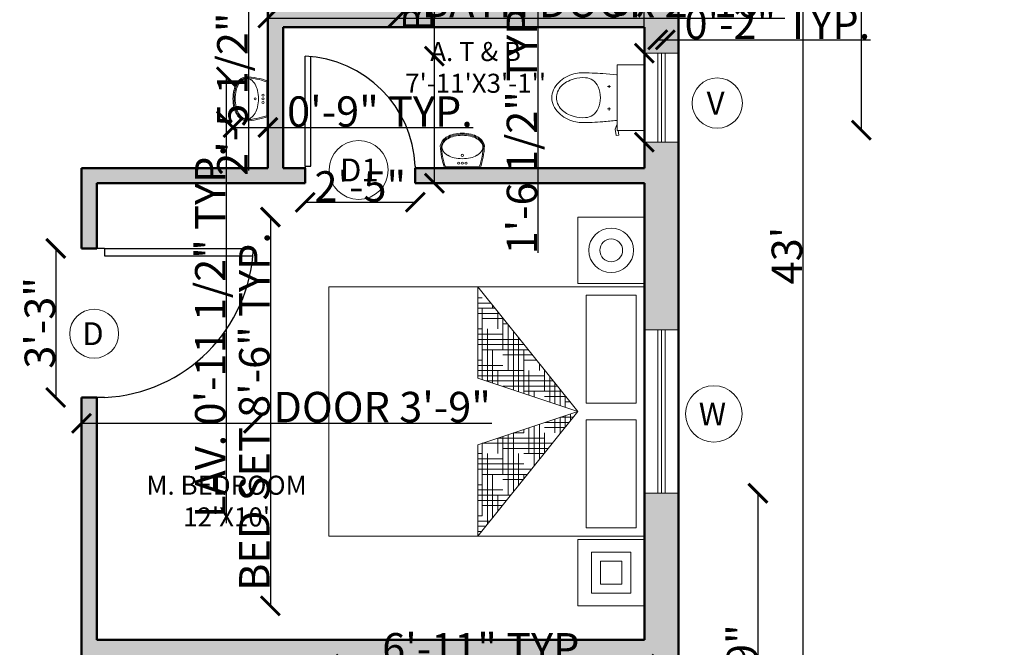
# Model space of a CAD drawing. Units: inches. Extents: x 2169 to 2662, y 1518 to 2151.
# Tile 5 of 6: x 2403 to 2662, y 1751 to 1916. Entities that reach past the tile are written whole.
import ezdxf

# ---------------------------------------------------------------- set-up
doc = ezdxf.new("R2010")
doc.units = ezdxf.units.IN
for name, color, linetype, lineweight in [('A-ANNO-DIMS', 2, 'Continuous', 18), ('A-ANNO-SYMB', 7, 'Continuous', 18), ('A-AREA-IDEN', 7, 'Continuous', 18), ('A-FLOR-FIXT', 9, 'Continuous', 18), ('A-FURN', 8, 'Continuous', 18), ('A-WALL-PATT', 30, 'Continuous', 13), ('Doors', 240, 'Continuous', 30), ('Walls', 7, 'Continuous', 50), ('Windows', 160, 'Continuous', 18)]:
    doc.layers.add(name, color=color, linetype=linetype, lineweight=lineweight)
doc.styles.get("Standard").update_dxf_attribs({"font": 'arial.ttf'})
doc.dimstyles.get("Standard").update_dxf_attribs({"dimtxt": 8, "dimasz": 5, "dimexe": 0.18, "dimexo": 0.0625, "dimgap": 0.09, "dimtad": 1, "dimdec": 1, "dimzin": 0, "dimdsep": 46, "dimlunit": 4, "dimtxsty": 'Standard', "dimblk": 'ARCHTICK', "dimcen": 0.09, "dimse1": 1, "dimse2": 1, "dimadec": 0, "dimazin": 0, "dimtfac": 1, "dimtdec": 1, "dimtofl": 0, "dimtmove": 0, "dimatfit": 3, "dimfxl": 1, "dimtolj": 1, "dimtzin": 0, "dimarcsym": 0})

# ---------------------------------------------------------------- blocks, each defined once
blk = doc.blocks.new('_ArchTick')
at = {"color": 0, "linetype": 'ByBlock', "const_width": 0.15}
blk.add_lwpolyline([(-0.5, -0.5), (0.5, 0.5)], dxfattribs=at)
blk = doc.blocks.new('*D3')
at = {"layer": 'A-ANNO-DIMS', "color": 0, "lineweight": -2, "transparency": 16777216}
blk.add_line((2608.61, 2111.6), (2608.61, 1595.6), dxfattribs=at)
at = {"layer": 'Defpoints', "color": 0, "transparency": 16777216}
for p in [(2575.74, 2111.6), (2575.98, 1595.6), (2608.61, 1595.6)]:
    blk.add_point(p, dxfattribs=at)
at = {"layer": 'A-ANNO-DIMS', "color": 0, "lineweight": -2, "transparency": 16777216, "xscale": 5, "yscale": 5, "zscale": 5}
for p, rotation in [((2608.61, 2111.6), 90), ((2608.61, 1595.6), 270)]:
    blk.add_blockref('_ArchTick', p, dxfattribs=dict(at, rotation=rotation))
at = {"layer": 'A-ANNO-DIMS', "color": 0, "transparency": 16777216, "insert": (2604.43, 1853.6), "char_height": 8, "attachment_point": 5, "rotation": 90}
blk.add_mtext("\\A1;43'", dxfattribs=at)
blk = doc.blocks.new('*X16')
at = {"color": 0}
for p, q in [((20.1875, 14.75), (20.1875, 14.7669)), ((20.199, 14.7812), (20.2772, 14.7812)), ((20.25, 14.8125), (20.2772, 14.8125)), ((20.1487, 14.7188), (20.2772, 14.7188)), ((20.1562, 14.625), (20.1562, 14.7281)), ((20.1739, 14.75), (20.2772, 14.75)), ((20.25, 14.3194), (20.25, 14.75)), ((20.0938, 14.375), (20.0938, 14.6504)), ((20.0984, 14.6562), (20.125, 14.6562)), ((20.1236, 14.6875), (20.25, 14.6875)), ((20.125, 14.5), (20.125, 14.6893)), ((20.0625, 14.2573), (20.0625, 14.6116)), ((20.125, 14.5938), (20.2772, 14.5938)), ((20.2188, 14.3091), (20.2188, 14.625)), ((20.25, 14.625), (20.2772, 14.625)), ((19.9979, 14.5312), (20.2772, 14.5312)), ((20.023, 14.5625), (20.2772, 14.5625)), ((20.0312, 14.2469), (20.0312, 14.5727)), ((19.9476, 14.4688), (20.125, 14.4688)), ((19.9727, 14.5), (20.25, 14.5)), ((20, 14.2366), (20, 14.5)), ((20.1875, 14.2987), (20.1875, 14.5)), ((19.9062, 14.375), (19.9062, 14.4174)), ((19.9225, 14.4375), (20, 14.4375)), ((20.125, 14.4062), (20.2772, 14.4062)), ((20.25, 14.4375), (20.2772, 14.4375)), ((19.875, 14.25), (19.875, 14.3785)), ((19.875, 14.3438), (20.2772, 14.3438)), ((19.9688, 14.2262), (19.9688, 14.375)), ((20, 14.375), (20.2772, 14.375)), ((20.1562, 14.2884), (20.1562, 14.375)), ((19.8125, 14.1744), (19.8125, 14.3008)), ((19.8219, 14.3125), (20.2291, 14.3125)), ((19.8438, 14.1848), (19.8438, 14.3397)), ((19.7716, 14.25), (20, 14.25)), ((19.7812, 14.1641), (19.7812, 14.262)), ((19.7967, 14.2812), (20.125, 14.2812)), ((19.9375, 14.2159), (19.9375, 14.25)), ((19.7213, 14.1875), (19.75, 14.1875)), ((19.7465, 14.2188), (19.875, 14.2188)), ((19.75, 14.1537), (19.75, 14.2231)), ((19.7188, 14.0726), (19.7188, 14.1136)), ((19.7018, 14.0938), (19.7786, 14.0938)), ((19.7269, 14.0625), (19.8728, 14.0625)), ((19.75, 14.0338), (19.75, 14.1032)), ((19.7812, 13.9949), (19.7812, 14.0929)), ((19.8125, 14), (19.8125, 14.0825)), ((19.9062, 13.8396), (19.9062, 14.0514)), ((19.752, 14.0312), (19.875, 14.0312)), ((19.875, 13.8784), (19.875, 14)), ((19.9375, 13.8007), (19.9375, 14.0411)), ((19.9688, 13.875), (19.9688, 14.0307)), ((20, 14), (20, 14.0204)), ((20, 14), (20.0614, 14)), ((20.0625, 13.6454), (20.0625, 13.9996)), ((20.0938, 13.625), (20.0938, 13.9893)), ((19.8275, 13.9375), (20.25, 13.9375)), ((19.875, 13.9688), (20.1557, 13.9688)), ((20.125, 13.75), (20.125, 13.9789)), ((20.1562, 13.875), (20.1562, 13.9686)), ((20.25, 13.5), (20.25, 13.9375)), ((19.8526, 13.9062), (20.125, 13.9062)), ((19.8777, 13.875), (20, 13.875)), ((20.0312, 13.6842), (20.0312, 13.875)), ((20.2188, 13.4511), (20.2188, 13.875)), ((20.25, 13.875), (20.2772, 13.875)), ((20, 13.8125), (20.2772, 13.8125)), ((20.125, 13.8438), (20.2772, 13.8438)), ((19.9532, 13.7812), (20.2772, 13.7812)), ((19.9783, 13.75), (20.25, 13.75)), ((20, 13.723), (20, 13.75)), ((20.0035, 13.7188), (20.125, 13.7188)), ((20.1875, 13.49), (20.1875, 13.75)), ((20.125, 13.6562), (20.2772, 13.6562)), ((20.25, 13.6875), (20.2772, 13.6875)), ((20.0789, 13.625), (20.2772, 13.625)), ((20.104, 13.5938), (20.2772, 13.5938)), ((20.1562, 13.5288), (20.1562, 13.625)), ((20.1292, 13.5625), (20.25, 13.5625)), ((20.2046, 13.4688), (20.2772, 13.4688)), ((20.25, 13.5), (20.2772, 13.5)), ((20.2297, 13.4375), (20.2772, 13.4375)), ((20.2549, 13.4062), (20.2772, 13.4062))]:
    blk.add_line(p, q, dxfattribs=at)
blk = doc.blocks.new('MAT-P13')
for p, q in [((-1.17, 0), (-1.17, -0.4)), ((-1.17, 0), (-0.77, 0)), ((-0.77, 0), (-0.77, -0.4)), ((-0.75, 0), (0.75, 0)), ((-0.75, 0), (-0.75, -1.9)), ((0.75, 0), (0.75, -1.9)), ((0.77, 0), (1.17, 0)), ((0.77, 0), (0.77, -0.4)), ((1.17, 0), (1.17, -0.4)), ((-0.7, -0.05), (-0.7, -0.35)), ((-0.7, -0.05), (-0.05, -0.05)), ((-0.05, -0.35), (-0.05, -0.05)), ((0.05, -0.05), (0.7, -0.05)), ((0.05, -0.35), (0.05, -0.05)), ((0.7, -0.05), (0.7, -0.35)), ((-0.7, -0.35), (-0.05, -0.35)), ((0.05, -0.35), (0.7, -0.35)), ((-1.17, -0.4), (-0.77, -0.4)), ((-0.75, -1.0034), (0, -0.4)), ((0, -0.4), (-0.75, -1.0034)), ((0, -0.4), (-0.2, -1.0034)), ((0, -0.4), (0.2, -1.0034)), ((0, -0.4), (0.75, -1.0034)), ((0.77, -0.4), (1.17, -0.4)), ((-0.75, -1.0034), (-0.2, -1.0034)), ((0.2, -1.0034), (0.75, -1.0034)), ((0.75, -1.9), (-0.75, -1.9))]:
    blk.add_line(p, q)
for points in [[(0.8468, -0.0814), (1.0932, -0.0814), (1.0932, -0.3186), (0.8468, -0.3186)], [(0.9015, -0.1361), (1.0385, -0.1361), (1.0385, -0.2639), (0.9015, -0.2639)]]:
    blk.add_lwpolyline(points, close=True)
for radius in [0.1342, 0.0686]:
    blk.add_circle((-0.97, -0.2), radius)
at = {"xscale": -1, "rotation": 90}
blk.add_blockref('*X16', (14.1285, 19.2738), dxfattribs=at)
blk = doc.blocks.new('toilet-1')
at = {"color": 0, "linetype": 'ByBlock'}
for p, q in [((-0.23, -0.02), (-0.23, -0.2116)), ((0.23, -0.02), (-0.23, -0.02)), ((0.23, -0.02), (0.23, -0.2116)), ((0.2633, -0.1997), (0.23, -0.2044)), ((0.266, -0.2187), (0.2633, -0.1997)), ((-0.23, -0.2116), (0.23, -0.2116)), ((-0.0889, -0.2683), (-0.0697, -0.2683)), ((-0.0793, -0.2587), (-0.0793, -0.2778)), ((0.0889, -0.2683), (0.0698, -0.2683)), ((0.0794, -0.2587), (0.0794, -0.2778)), ((0.1917, -0.2144), (0.2206, -0.225)), ((0.2206, -0.225), (0.266, -0.2187)), ((0, -0.6382), (0, -0.6382))]:
    blk.add_line(p, q, dxfattribs=at)
for centre, radius, start, end in [((3.5272, -0.6239), 3.7093, 173.69251, 175.15926), ((-3.527, -0.624), 3.7093, 4.84131, 6.31706), ((1.7368, -0.4519), 1.9109, 175.76982, 180.37578), ((-0.0312, -0.4465), 0.1114, 113.89968, 145.1485), ((0, -0.5169), 0.1884, 66.09393, 113.90607), ((0.0312, -0.4465), 0.1114, 34.8515, 66.10032), ((-1.7366, -0.4519), 1.9109, 359.62422, 4.23018), ((-0.0408, -0.4398), 0.0996, 145.14967, 175.88096), ((0.0409, -0.4398), 0.0996, 4.11904, 34.85033), ((0.0353, -0.463), 0.2093, 180.37466, 194.33753), ((0.0981, -0.4497), 0.2389, 175.88621, 195.59308), ((-0.098, -0.4497), 0.2389, 344.40692, 4.11379), ((-0.0351, -0.463), 0.2093, 345.6614, 359.62427), ((0.055, -0.458), 0.2297, 194.33532, 209.62204), ((0.0961, -0.4503), 0.2369, 195.59686, 209.37705), ((-0.096, -0.4503), 0.2369, 330.62295, 344.40314), ((-0.0548, -0.458), 0.2297, 330.37879, 345.66551), ((0.0647, -0.4524), 0.2409, 209.62726, 224.54888), ((0.0232, -0.4913), 0.1532, 209.38715, 226.54376), ((0.0178, -0.4986), 0.1751, 224.55199, 245.714), ((0.0152, -0.4997), 0.1416, 226.55015, 246.55272), ((-0.0151, -0.4997), 0.1416, 293.44728, 313.44985), ((-0.0176, -0.4986), 0.1751, 294.28649, 315.4485), ((-0.0231, -0.4913), 0.1532, 313.45624, 330.61285), ((-0.0645, -0.4524), 0.2409, 315.45042, 330.37204), ((0.0004, -0.538), 0.132, 245.58449, 269.87817), ((0, -0.5347), 0.1034, 246.54933, 270.0042), ((0, -0.5347), 0.1034, 269.9958, 293.45067), ((-0.0002, -0.538), 0.132, 270.12162, 294.4153)]:
    blk.add_arc(centre, radius, start, end, dxfattribs=at)
blk = doc.blocks.new('wash-3')
at = {"color": 0, "linetype": 'ByBlock'}
blk.add_line((0.23, -0.015), (-0.23, -0.015), dxfattribs=at)
for centre in [(-0.05, -0.066), (0, -0.066), (0.05, -0.066), (0, -0.172)]:
    blk.add_circle(centre, 0.0148, dxfattribs=at)
for centre, radius, start, end in [((0.69, -0.34), 0.991, 159.941, 177.839), ((0.69, -0.34), 0.976, 160.5399, 177.7326), ((0, -0.61), 0.483, 90, 103.3619), ((0, -0.61), 0.483, 76.6381, 90), ((-0.69, -0.34), 0.976, 2.2674, 19.4601), ((-0.69, -0.34), 0.991, 2.161, 20.059), ((-0.183, -0.286), 0.095, 144.1588, 180), ((-0.096, -0.349), 0.203, 119.8322, 144.1588), ((-0.038, -0.45), 0.319, 103.3619, 119.8322), ((0.038, -0.45), 0.319, 60.1678, 76.6381), ((0.096, -0.349), 0.203, 35.8412, 60.1678), ((0.183, -0.286), 0.095, 0, 35.8412), ((-0.12, -0.265), 0.184, 191.7424, 233.4191), ((-0.12, -0.265), 0.169, 192.3358, 233.361), ((-0.183, -0.286), 0.095, 180, 215.8412), ((-0.096, -0.223), 0.203, 215.8412, 240.1678), ((-0.096, -0.223), 0.217, 234.8176, 240.1678), ((-0.038, -0.122), 0.319, 240.1678, 256.6381), ((0.038, -0.122), 0.319, 283.3619, 299.8322), ((0.096, -0.223), 0.203, 299.8322, 324.1588), ((0.096, -0.223), 0.217, 299.8322, 305.1824), ((0.12, -0.265), 0.169, 306.639, 347.6642), ((0.12, -0.265), 0.184, 306.5809, 348.2576), ((0.183, -0.286), 0.095, 324.1588, 0), ((-0.096, -0.223), 0.232, 234.7719, 240.1678), ((-0.038, -0.122), 0.348, 240.1678, 256.6381), ((-0.038, -0.122), 0.333, 240.1678, 256.6381), ((0, 0.038), 0.513, 256.6381, 270), ((0, 0.038), 0.498, 256.6381, 270), ((0, 0.038), 0.483, 256.6381, 270), ((0, 0.038), 0.483, 270, 283.3619), ((0, 0.038), 0.498, 270, 283.3619), ((0, 0.038), 0.513, 270, 283.3619), ((0.038, -0.122), 0.333, 283.3619, 299.8322), ((0.038, -0.122), 0.348, 283.3619, 299.8322), ((0.096, -0.223), 0.232, 299.8322, 305.2281)]:
    blk.add_arc(centre, radius, start, end, dxfattribs=at)
blk = doc.blocks.new('AP0B05')
for p, q in [((35, 100), (35, 880)), ((75, 100), (75, 878.9)), ((35, 100), (35, -20)), ((815, 100), (815, -20))]:
    blk.add_line(p, q)
blk.add_lwpolyline([(35, 100), (75, 100)])
blk.add_arc((-2.4, 62.6), 818.3, 2.6212, 87.3788)
blk = doc.blocks.new('GLAZING-43IN')
for p, q in [((-21.5, 1), (21.5, 1)), ((-21.5, 0), (21.5, 0)), ((-21.5, -1), (21.5, -1))]:
    blk.add_line(p, q)
blk = doc.blocks.new('GLAZING-SHORT')
for p, q in [((-1, -11.72), (-1, 11.72)), ((0, -11.72), (0, 11.72)), ((1, -11.72), (1, 11.72))]:
    blk.add_line(p, q)
blk = doc.blocks.new('OPENING-TAG-W')
blk.add_circle((0, 0), 7.42)
blk.add_text('W', height=6).set_placement((-3.96, -3))
blk = doc.blocks.new('OPENING-TAG-D')
blk.add_circle((0, 0), 6.43)
blk.add_text('D', height=6).set_placement((-3.13, -3))
blk = doc.blocks.new('OPENING-TAG-V')
blk.add_circle((0, 0), 6.61)
blk.add_text('V', height=6).set_placement((-2.78, -3))
blk = doc.blocks.new('OPENING-TAG-D1')
blk.add_circle((0, 0), 7.74)
blk.add_text('D1', height=6).set_placement((-4.91, -3.01))
blk = doc.blocks.new('*D27')
at = {"layer": 'A-ANNO-DIMS', "color": 0, "lineweight": -2, "transparency": 16777216}
for p, q in [((2566.96, 1906.83), (2566.96, 2079.95)), ((2566.96, 1883.38), (2566.96, 1906.83))]:
    blk.add_line(p, q, dxfattribs=at)
at = {"layer": 'Defpoints', "color": 0, "transparency": 16777216}
for p in [(2566.96, 1906.83), (2570.48, 1906.83), (2570.48, 1883.38)]:
    blk.add_point(p, dxfattribs=at)
at = {"layer": 'A-ANNO-DIMS', "color": 0, "lineweight": -2, "transparency": 16777216, "xscale": 5, "yscale": 5, "zscale": 5}
for p, rotation in [((2566.96, 1906.83), 90), ((2566.96, 1883.38), 270)]:
    blk.add_blockref('_ArchTick', p, dxfattribs=dict(at, rotation=rotation))
at = {"layer": 'A-ANNO-DIMS', "color": 0, "transparency": 16777216, "insert": (2562.73, 1995.89), "char_height": 8, "attachment_point": 5, "rotation": 90}
blk.add_mtext('\\A1;SHORT WINDOW 1\'-11 1/2" TYP.', dxfattribs=at)
blk = doc.blocks.new('*D28')
at = {"layer": 'A-ANNO-DIMS', "color": 0, "lineweight": -2, "transparency": 16777216}
for p, q in [((2570.48, 1910.34), (2572.48, 1910.34)), ((2572.48, 1910.34), (2626.42, 1910.34))]:
    blk.add_line(p, q, dxfattribs=at)
at = {"layer": 'Defpoints', "color": 0, "transparency": 16777216}
for p in [(2572.48, 1910.34), (2570.48, 1906.83), (2572.48, 1906.83)]:
    blk.add_point(p, dxfattribs=at)
at = {"layer": 'A-ANNO-DIMS', "color": 0, "lineweight": -2, "transparency": 16777216, "xscale": 5, "yscale": 5, "zscale": 5, "rotation": 180}
blk.add_blockref('_ArchTick', (2570.48, 1910.34), dxfattribs=at)
at = {"layer": 'A-ANNO-DIMS', "color": 0, "lineweight": -2, "transparency": 16777216, "xscale": 5, "yscale": 5, "zscale": 5}
blk.add_blockref('_ArchTick', (2572.48, 1910.34), dxfattribs=at)
at = {"layer": 'A-ANNO-DIMS', "color": 0, "transparency": 16777216, "insert": (2601.95, 1914.52), "char_height": 8, "attachment_point": 5}
blk.add_mtext('\\A1;0\'-2" TYP.', dxfattribs=at)
blk = doc.blocks.new('*D33')
at = {"layer": 'A-ANNO-DIMS', "color": 0, "lineweight": -2, "transparency": 16777216}
for p, q in [((2467.98, 1916.03), (2502.05, 1916.03)), ((2502.05, 1916.03), (2603.9, 1916.03))]:
    blk.add_line(p, q, dxfattribs=at)
at = {"layer": 'Defpoints', "color": 0, "transparency": 16777216}
for p in [(2467.98, 1921.14), (2502.05, 1921.14), (2502.05, 1916.03)]:
    blk.add_point(p, dxfattribs=at)
at = {"layer": 'A-ANNO-DIMS', "color": 0, "lineweight": -2, "transparency": 16777216, "xscale": 5, "yscale": 5, "zscale": 5, "rotation": 180}
blk.add_blockref('_ArchTick', (2467.98, 1916.03), dxfattribs=at)
at = {"layer": 'A-ANNO-DIMS', "color": 0, "lineweight": -2, "transparency": 16777216, "xscale": 5, "yscale": 5, "zscale": 5}
blk.add_blockref('_ArchTick', (2502.05, 1916.03), dxfattribs=at)
at = {"layer": 'A-ANNO-DIMS', "color": 0, "transparency": 16777216, "insert": (2555.47, 1920.26), "char_height": 8, "attachment_point": 5}
blk.add_mtext('\\A1;BATH DOOR 2\'-10"', dxfattribs=at)
blk = doc.blocks.new('*D34')
at = {"layer": 'A-ANNO-DIMS', "color": 0, "lineweight": -2, "transparency": 16777216}
for p, q in [((2462.86, 1950.67), (2462.86, 1921.14)), ((2462.86, 1921.14), (2462.86, 1875.92))]:
    blk.add_line(p, q, dxfattribs=at)
at = {"layer": 'Defpoints', "color": 0, "transparency": 16777216}
for p in [(2467.98, 1950.67), (2462.86, 1921.14), (2467.98, 1921.14)]:
    blk.add_point(p, dxfattribs=at)
at = {"layer": 'A-ANNO-DIMS', "color": 0, "lineweight": -2, "transparency": 16777216, "xscale": 5, "yscale": 5, "zscale": 5}
for p, rotation in [((2462.86, 1950.67), 90), ((2462.86, 1921.14), 270)]:
    blk.add_blockref('_ArchTick', p, dxfattribs=dict(at, rotation=rotation))
at = {"layer": 'A-ANNO-DIMS', "color": 0, "transparency": 16777216, "insert": (2458.64, 1896.03), "char_height": 8, "attachment_point": 5, "rotation": 90}
blk.add_mtext('\\A1;2\'-5 1/2"', dxfattribs=at)
blk = doc.blocks.new('*D35')
at = {"layer": 'A-ANNO-DIMS', "color": 0, "lineweight": -2, "transparency": 16777216}
for p, q in [((2418.98, 1809.52), (2464.19, 1809.52)), ((2464.19, 1809.52), (2526.87, 1809.52))]:
    blk.add_line(p, q, dxfattribs=at)
at = {"layer": 'Defpoints', "color": 0, "transparency": 16777216}
for p in [(2418.98, 1816.31), (2464.19, 1816.31), (2464.19, 1809.52)]:
    blk.add_point(p, dxfattribs=at)
at = {"layer": 'A-ANNO-DIMS', "color": 0, "lineweight": -2, "transparency": 16777216, "xscale": 5, "yscale": 5, "zscale": 5, "rotation": 180}
blk.add_blockref('_ArchTick', (2418.98, 1809.52), dxfattribs=at)
at = {"layer": 'A-ANNO-DIMS', "color": 0, "lineweight": -2, "transparency": 16777216, "xscale": 5, "yscale": 5, "zscale": 5}
blk.add_blockref('_ArchTick', (2464.19, 1809.52), dxfattribs=at)
at = {"layer": 'A-ANNO-DIMS', "color": 0, "transparency": 16777216, "insert": (2498.03, 1813.76), "char_height": 8, "attachment_point": 5}
blk.add_mtext('\\A1;DOOR 3\'-9"', dxfattribs=at)
blk = doc.blocks.new('*D36')
at = {"layer": 'A-ANNO-DIMS', "color": 0, "lineweight": -2, "transparency": 16777216}
blk.add_line((2412.19, 1855.49), (2412.19, 1816.31), dxfattribs=at)
at = {"layer": 'Defpoints', "color": 0, "transparency": 16777216}
for p in [(2418.98, 1855.49), (2412.19, 1816.31), (2418.98, 1816.31)]:
    blk.add_point(p, dxfattribs=at)
at = {"layer": 'A-ANNO-DIMS', "color": 0, "lineweight": -2, "transparency": 16777216, "xscale": 5, "yscale": 5, "zscale": 5}
for p, rotation in [((2412.19, 1855.49), 90), ((2412.19, 1816.31), 270)]:
    blk.add_blockref('_ArchTick', p, dxfattribs=dict(at, rotation=rotation))
at = {"layer": 'A-ANNO-DIMS', "color": 0, "transparency": 16777216, "insert": (2408.02, 1835.9), "char_height": 8, "attachment_point": 5, "rotation": 90}
blk.add_mtext('\\A1;3\'-3"', dxfattribs=at)
blk = doc.blocks.new('*D39')
at = {"layer": 'A-ANNO-DIMS', "color": 0, "lineweight": -2, "transparency": 16777216}
for p, q in [((2511.76, 1906), (2511.76, 2020.27)), ((2511.76, 1872.6), (2511.76, 1906))]:
    blk.add_line(p, q, dxfattribs=at)
at = {"layer": 'Defpoints', "color": 0, "transparency": 16777216}
for p in [(2506.75, 1906), (2511.76, 1906), (2506.75, 1872.6)]:
    blk.add_point(p, dxfattribs=at)
at = {"layer": 'A-ANNO-DIMS', "color": 0, "lineweight": -2, "transparency": 16777216, "xscale": 5, "yscale": 5, "zscale": 5}
for p, rotation in [((2511.76, 1906), 90), ((2511.76, 1872.6), 270)]:
    blk.add_blockref('_ArchTick', p, dxfattribs=dict(at, rotation=rotation))
at = {"layer": 'A-ANNO-DIMS', "color": 0, "transparency": 16777216, "insert": (2507.53, 1965.63), "char_height": 8, "attachment_point": 5, "rotation": 90}
blk.add_mtext('\\A1;BATH DOOR 2\'-9 1/2"', dxfattribs=at)
blk = doc.blocks.new('*D40')
at = {"layer": 'A-ANNO-DIMS', "color": 0, "lineweight": -2, "transparency": 16777216}
blk.add_line((2477.81, 1867.6), (2506.75, 1867.6), dxfattribs=at)
at = {"layer": 'Defpoints', "color": 0, "transparency": 16777216}
for p in [(2477.81, 1872.6), (2506.75, 1872.6), (2506.75, 1867.6)]:
    blk.add_point(p, dxfattribs=at)
at = {"layer": 'A-ANNO-DIMS', "color": 0, "lineweight": -2, "transparency": 16777216, "xscale": 5, "yscale": 5, "zscale": 5, "rotation": 180}
blk.add_blockref('_ArchTick', (2477.81, 1867.6), dxfattribs=at)
at = {"layer": 'A-ANNO-DIMS', "color": 0, "lineweight": -2, "transparency": 16777216, "xscale": 5, "yscale": 5, "zscale": 5}
blk.add_blockref('_ArchTick', (2506.75, 1867.6), dxfattribs=at)
at = {"layer": 'A-ANNO-DIMS', "color": 0, "transparency": 16777216, "insert": (2492.28, 1871.77), "char_height": 8, "attachment_point": 5}
blk.add_mtext('\\A1;2\'-5"', dxfattribs=at)
blk = doc.blocks.new('*D43')
at = {"layer": 'A-ANNO-DIMS', "color": 0, "lineweight": -2, "transparency": 16777216}
blk.add_line((2468.65, 1863.71), (2468.65, 1761.5), dxfattribs=at)
at = {"layer": 'Defpoints', "color": 0, "transparency": 16777216}
for p in [(2483.98, 1863.71), (2468.65, 1761.5), (2483.98, 1761.5)]:
    blk.add_point(p, dxfattribs=at)
at = {"layer": 'A-ANNO-DIMS', "color": 0, "lineweight": -2, "transparency": 16777216, "xscale": 5, "yscale": 5, "zscale": 5}
for p, rotation in [((2468.65, 1863.71), 90), ((2468.65, 1761.5), 270)]:
    blk.add_blockref('_ArchTick', p, dxfattribs=dict(at, rotation=rotation))
at = {"layer": 'A-ANNO-DIMS', "color": 0, "transparency": 16777216, "insert": (2464.42, 1812.6), "char_height": 8, "attachment_point": 5, "rotation": 90}
blk.add_mtext('\\A1;BED SET 8\'-6" TYP.', dxfattribs=at)
blk = doc.blocks.new('*D44')
at = {"layer": 'A-ANNO-DIMS', "color": 0, "lineweight": -2, "transparency": 16777216}
blk.add_line((2483.98, 1746.17), (2566.98, 1746.17), dxfattribs=at)
at = {"layer": 'Defpoints', "color": 0, "transparency": 16777216}
for p in [(2483.98, 1761.5), (2566.98, 1761.5), (2566.98, 1746.17)]:
    blk.add_point(p, dxfattribs=at)
at = {"layer": 'A-ANNO-DIMS', "color": 0, "lineweight": -2, "transparency": 16777216, "xscale": 5, "yscale": 5, "zscale": 5, "rotation": 180}
blk.add_blockref('_ArchTick', (2483.98, 1746.17), dxfattribs=at)
at = {"layer": 'A-ANNO-DIMS', "color": 0, "lineweight": -2, "transparency": 16777216, "xscale": 5, "yscale": 5, "zscale": 5}
blk.add_blockref('_ArchTick', (2566.98, 1746.17), dxfattribs=at)
at = {"layer": 'A-ANNO-DIMS', "color": 0, "transparency": 16777216, "insert": (2525.48, 1750.34), "char_height": 8, "attachment_point": 5}
blk.add_mtext('\\A1;6\'-11" TYP.', dxfattribs=at)
blk = doc.blocks.new('*D49')
at = {"layer": 'A-ANNO-DIMS', "color": 0, "lineweight": -2, "transparency": 16777216}
for p, q in [((2542.64, 1922.5), (2566.98, 1922.5)), ((2566.98, 1922.5), (2661.61, 1922.5))]:
    blk.add_line(p, q, dxfattribs=at)
at = {"layer": 'Defpoints', "color": 0, "transparency": 16777216}
for p in [(2542.64, 1926.15), (2566.98, 1926.15), (2566.98, 1922.5)]:
    blk.add_point(p, dxfattribs=at)
at = {"layer": 'A-ANNO-DIMS', "color": 0, "lineweight": -2, "transparency": 16777216, "xscale": 5, "yscale": 5, "zscale": 5, "rotation": 180}
blk.add_blockref('_ArchTick', (2542.64, 1922.5), dxfattribs=at)
at = {"layer": 'A-ANNO-DIMS', "color": 0, "lineweight": -2, "transparency": 16777216, "xscale": 5, "yscale": 5, "zscale": 5}
blk.add_blockref('_ArchTick', (2566.98, 1922.5), dxfattribs=at)
at = {"layer": 'A-ANNO-DIMS', "color": 0, "transparency": 16777216, "insert": (2616.79, 1926.72), "char_height": 8, "attachment_point": 5}
blk.add_mtext('\\A1;WC 2\'-0 1/2" TYP.', dxfattribs=at)
blk = doc.blocks.new('*D50')
at = {"layer": 'A-ANNO-DIMS', "color": 0, "lineweight": -2, "transparency": 16777216}
for p, q in [((2538.99, 1944.71), (2538.99, 1926.15)), ((2538.99, 1926.15), (2538.99, 1854.31))]:
    blk.add_line(p, q, dxfattribs=at)
at = {"layer": 'Defpoints', "color": 0, "transparency": 16777216}
for p in [(2542.64, 1944.71), (2538.99, 1926.15), (2542.64, 1926.15)]:
    blk.add_point(p, dxfattribs=at)
at = {"layer": 'A-ANNO-DIMS', "color": 0, "lineweight": -2, "transparency": 16777216, "xscale": 5, "yscale": 5, "zscale": 5}
for p, rotation in [((2538.99, 1944.71), 90), ((2538.99, 1926.15), 270)]:
    blk.add_blockref('_ArchTick', p, dxfattribs=dict(at, rotation=rotation))
at = {"layer": 'A-ANNO-DIMS', "color": 0, "transparency": 16777216, "insert": (2534.77, 1887.73), "char_height": 8, "attachment_point": 5, "rotation": 90}
blk.add_mtext('\\A1;1\'-6 1/2" TYP.', dxfattribs=at)
blk = doc.blocks.new('*D51')
at = {"layer": 'A-ANNO-DIMS', "color": 0, "lineweight": -2, "transparency": 16777216}
for p, q in [((2457.05, 1900.61), (2457.05, 1889.01)), ((2457.05, 1889.01), (2457.05, 1783.23))]:
    blk.add_line(p, q, dxfattribs=at)
at = {"layer": 'Defpoints', "color": 0, "transparency": 16777216}
for p in [(2458.79, 1900.61), (2457.05, 1889.01), (2458.79, 1889.01)]:
    blk.add_point(p, dxfattribs=at)
at = {"layer": 'A-ANNO-DIMS', "color": 0, "lineweight": -2, "transparency": 16777216, "xscale": 5, "yscale": 5, "zscale": 5}
for p, rotation in [((2457.05, 1900.61), 90), ((2457.05, 1889.01), 270)]:
    blk.add_blockref('_ArchTick', p, dxfattribs=dict(at, rotation=rotation))
at = {"layer": 'A-ANNO-DIMS', "color": 0, "transparency": 16777216, "insert": (2452.83, 1833.62), "char_height": 8, "attachment_point": 5, "rotation": 90}
blk.add_mtext('\\A1;LAV. 0\'-11 1/2" TYP.', dxfattribs=at)
blk = doc.blocks.new('*D52')
at = {"layer": 'A-ANNO-DIMS', "color": 0, "lineweight": -2, "transparency": 16777216}
for p, q in [((2458.79, 1887.27), (2467.98, 1887.27)), ((2467.98, 1887.27), (2521.92, 1887.27))]:
    blk.add_line(p, q, dxfattribs=at)
at = {"layer": 'Defpoints', "color": 0, "transparency": 16777216}
for p in [(2458.79, 1889.01), (2467.98, 1889.01), (2467.98, 1887.27)]:
    blk.add_point(p, dxfattribs=at)
at = {"layer": 'A-ANNO-DIMS', "color": 0, "lineweight": -2, "transparency": 16777216, "xscale": 5, "yscale": 5, "zscale": 5, "rotation": 180}
blk.add_blockref('_ArchTick', (2458.79, 1887.27), dxfattribs=at)
at = {"layer": 'A-ANNO-DIMS', "color": 0, "lineweight": -2, "transparency": 16777216, "xscale": 5, "yscale": 5, "zscale": 5}
blk.add_blockref('_ArchTick', (2467.98, 1887.27), dxfattribs=at)
at = {"layer": 'A-ANNO-DIMS', "color": 0, "transparency": 16777216, "insert": (2497.45, 1891.45), "char_height": 8, "attachment_point": 5}
blk.add_mtext('\\A1;0\'-9" TYP.', dxfattribs=at)
blk = doc.blocks.new('*D55')
at = {"layer": 'A-ANNO-DIMS', "color": 0, "lineweight": -2, "transparency": 16777216}
blk.add_line((2462.45, 2141.45), (2522.45, 2141.45), dxfattribs=at)
at = {"layer": 'Defpoints', "color": 0, "transparency": 16777216}
for p in [(2522.45, 2141.45), (2462.45, 1604.6), (2522.45, 1604.6)]:
    blk.add_point(p, dxfattribs=at)
at = {"layer": 'A-ANNO-DIMS', "color": 0, "lineweight": -2, "transparency": 16777216, "xscale": 5, "yscale": 5, "zscale": 5, "rotation": 180}
blk.add_blockref('_ArchTick', (2462.45, 2141.45), dxfattribs=at)
at = {"layer": 'A-ANNO-DIMS', "color": 0, "lineweight": -2, "transparency": 16777216, "xscale": 5, "yscale": 5, "zscale": 5}
blk.add_blockref('_ArchTick', (2522.45, 2141.45), dxfattribs=at)
at = {"layer": 'A-ANNO-DIMS', "color": 0, "transparency": 16777216, "insert": (2492.45, 2145.63), "char_height": 8, "attachment_point": 5}
blk.add_mtext('\\A1;5\'-0"', dxfattribs=at)
blk = doc.blocks.new('*D62')
at = {"layer": 'A-ANNO-DIMS', "color": 0, "lineweight": -2, "transparency": 16777216}
blk.add_line((2596.83, 1791.1), (2596.83, 1698.1), dxfattribs=at)
at = {"layer": 'Defpoints', "color": 0, "transparency": 16777216}
for p in [(2566.98, 1791.1), (2566.98, 1698.1), (2596.83, 1698.1)]:
    blk.add_point(p, dxfattribs=at)
at = {"layer": 'A-ANNO-DIMS', "color": 0, "lineweight": -2, "transparency": 16777216, "xscale": 5, "yscale": 5, "zscale": 5}
for p, rotation in [((2596.83, 1791.1), 90), ((2596.83, 1698.1), 270)]:
    blk.add_blockref('_ArchTick', p, dxfattribs=dict(at, rotation=rotation))
at = {"layer": 'A-ANNO-DIMS', "color": 0, "transparency": 16777216, "insert": (2592.65, 1744.6), "char_height": 8, "attachment_point": 5, "rotation": 90}
blk.add_mtext('\\A1;7\'-9"', dxfattribs=at)
blk = doc.blocks.new('*D73')
at = {"layer": 'A-ANNO-DIMS', "color": 0, "lineweight": -2, "transparency": 16777216}
blk.add_line((2624.02, 1886.6), (2624.02, 1978.6), dxfattribs=at)
at = {"layer": 'Defpoints', "color": 0, "transparency": 16777216}
for p in [(2369.77, 1978.6), (2624.02, 1978.6), (2370.48, 1886.6)]:
    blk.add_point(p, dxfattribs=at)
at = {"layer": 'A-ANNO-DIMS', "color": 0, "lineweight": -2, "transparency": 16777216, "xscale": 5, "yscale": 5, "zscale": 5}
for p, rotation in [((2624.02, 1978.6), 90), ((2624.02, 1886.6), 270)]:
    blk.add_blockref('_ArchTick', p, dxfattribs=dict(at, rotation=rotation))
at = {"layer": 'A-ANNO-DIMS', "color": 0, "transparency": 16777216, "insert": (2619.84, 1932.6), "char_height": 8, "attachment_point": 5, "rotation": 90}
blk.add_mtext('\\A1;7\'-8"', dxfattribs=at)
blk = doc.blocks.new('*D77')
at = {"layer": 'A-ANNO-DIMS', "color": 0, "lineweight": -2, "transparency": 16777216}
blk.add_line((2566.98, 1525.75), (2523.78, 1525.75), dxfattribs=at)
at = {"layer": 'Defpoints', "color": 0, "transparency": 16777216}
for p in [(2523.78, 1876.6), (2566.98, 1876.6), (2523.78, 1525.75)]:
    blk.add_point(p, dxfattribs=at)
at = {"layer": 'A-ANNO-DIMS', "color": 0, "lineweight": -2, "transparency": 16777216, "xscale": 5, "yscale": 5, "zscale": 5, "rotation": 180}
blk.add_blockref('_ArchTick', (2523.78, 1525.75), dxfattribs=at)
at = {"layer": 'A-ANNO-DIMS', "color": 0, "lineweight": -2, "transparency": 16777216, "xscale": 5, "yscale": 5, "zscale": 5}
blk.add_blockref('_ArchTick', (2566.98, 1525.75), dxfattribs=at)
at = {"layer": 'A-ANNO-DIMS', "color": 0, "transparency": 16777216, "insert": (2545.38, 1529.93), "char_height": 8, "attachment_point": 5}
blk.add_mtext('\\A1;3\'-7"', dxfattribs=at)
blk = doc.blocks.new('*D78')
at = {"layer": 'A-ANNO-DIMS', "color": 0, "lineweight": -2, "transparency": 16777216}
for p, q in [((2393.13, 1748.6), (2393.13, 1792.94)), ((2393.13, 1729.93), (2393.13, 1748.6))]:
    blk.add_line(p, q, dxfattribs=at)
at = {"layer": 'Defpoints', "color": 0, "transparency": 16777216}
for p in [(2393.13, 1748.6), (2422.98, 1748.6), (2422.98, 1729.93)]:
    blk.add_point(p, dxfattribs=at)
at = {"layer": 'A-ANNO-DIMS', "color": 0, "lineweight": -2, "transparency": 16777216, "xscale": 5, "yscale": 5, "zscale": 5}
for p, rotation in [((2393.13, 1748.6), 90), ((2393.13, 1729.93), 270)]:
    blk.add_blockref('_ArchTick', p, dxfattribs=dict(at, rotation=rotation))
at = {"layer": 'A-ANNO-DIMS', "color": 0, "transparency": 16777216, "insert": (2388.9, 1773.27), "char_height": 8, "attachment_point": 5, "rotation": 90}
blk.add_mtext('\\A1;1\'-6 1/2"', dxfattribs=at)
blk = doc.blocks.new('*D79')
at = {"layer": 'A-ANNO-DIMS', "color": 0, "lineweight": -2, "transparency": 16777216}
for p, q in [((2393.13, 1872.6), (2393.13, 1898.3)), ((2393.13, 1855.49), (2393.13, 1872.6))]:
    blk.add_line(p, q, dxfattribs=at)
at = {"layer": 'Defpoints', "color": 0, "transparency": 16777216}
for p in [(2393.13, 1872.6), (2422.98, 1872.6), (2422.98, 1855.49)]:
    blk.add_point(p, dxfattribs=at)
at = {"layer": 'A-ANNO-DIMS', "color": 0, "lineweight": -2, "transparency": 16777216, "xscale": 5, "yscale": 5, "zscale": 5}
for p, rotation in [((2393.13, 1872.6), 90), ((2393.13, 1855.49), 270)]:
    blk.add_blockref('_ArchTick', p, dxfattribs=dict(at, rotation=rotation))
at = {"layer": 'A-ANNO-DIMS', "color": 0, "transparency": 16777216, "insert": (2388.95, 1887.95), "char_height": 8, "attachment_point": 5, "rotation": 90}
blk.add_mtext('\\A1;1\'-5"', dxfattribs=at)
blk = doc.blocks.new('*D86')
at = {"layer": 'A-ANNO-DIMS', "color": 0, "lineweight": -2, "transparency": 16777216}
for p, q in [((2471.98, 1525.75), (2477.81, 1525.75)), ((2477.81, 1525.75), (2504.25, 1525.75))]:
    blk.add_line(p, q, dxfattribs=at)
at = {"layer": 'Defpoints', "color": 0, "transparency": 16777216}
for p in [(2471.98, 1876.6), (2477.81, 1876.6), (2477.81, 1525.75)]:
    blk.add_point(p, dxfattribs=at)
at = {"layer": 'A-ANNO-DIMS', "color": 0, "lineweight": -2, "transparency": 16777216, "xscale": 5, "yscale": 5, "zscale": 5, "rotation": 180}
blk.add_blockref('_ArchTick', (2471.98, 1525.75), dxfattribs=at)
at = {"layer": 'A-ANNO-DIMS', "color": 0, "lineweight": -2, "transparency": 16777216, "xscale": 5, "yscale": 5, "zscale": 5}
blk.add_blockref('_ArchTick', (2477.81, 1525.75), dxfattribs=at)
at = {"layer": 'A-ANNO-DIMS', "color": 0, "transparency": 16777216, "insert": (2493.53, 1529.93), "char_height": 8, "attachment_point": 5}
blk.add_mtext('\\A1;0\'-6"', dxfattribs=at)

msp = doc.modelspace()

# ---------------------------------------------------------------- hatches: boundary and pattern name
at = {"layer": 'A-WALL-PATT', "transparency": 33554585}
h = msp.add_hatch(color=256, dxfattribs=at)
h.dxf.hatch_style = 1
h.paths.add_polyline_path([(2575.98, 2111.6), (2263.98, 2111.6), (2263.98, 2066.68), (2272.98, 2066.68), (2272.98, 2102.6), (2418.98, 2102.6), (2418.98, 1982.6), (2413.75, 1982.6), (2413.75, 1978.6), (2418.98, 1978.6), (2418.98, 1954.6), (2429.26, 1954.6), (2429.26, 1958.6), (2422.98, 1958.6), (2422.98, 2102.6), (2566.98, 2102.6), (2566.98, 2052.1), (2575.98, 2052.1)])
h.paths.add_polyline_path([(2575.98, 2009.1), (2566.98, 2009.1), (2566.98, 1997.84), (2566.98, 1958.6), (2467.98, 1958.6), (2467.98, 1950.67), (2471.98, 1950.67), (2471.98, 1954.6), (2566.98, 1954.6), (2566.98, 1947.83), (2575.98, 1947.83)])
h.paths.add_polyline_path([(2272.98, 2023.68), (2263.98, 2023.68), (2263.98, 1944.7), (2272.98, 1944.7), (2272.98, 1978.6), (2369.77, 1978.6), (2369.77, 1982.6), (2272.98, 1982.6)])
h.paths.add_polyline_path([(2272.98, 1882.6), (2370.48, 1882.6), (2370.48, 1886.6), (2272.98, 1886.6), (2272.98, 1921.26), (2263.98, 1921.26), (2263.98, 1841.55), (2272.98, 1841.55)])
h.paths.add_polyline_path([(2272.98, 1798.55), (2263.98, 1798.55), (2263.98, 1689.49), (2272.98, 1689.49)])
h.paths.add_polyline_path([(2272.98, 1646.49), (2263.98, 1646.49), (2263.98, 1595.6), (2281.85, 1595.6), (2281.85, 1604.6), (2272.98, 1604.6)])
h.paths.add_polyline_path([(2342.72, 1600.02), (2342.72, 1604.6), (2324.85, 1604.6), (2324.85, 1595.6), (2342.72, 1595.6)])
h.paths.add_polyline_path([(2462.45, 1604.6), (2408.92, 1604.6), (2408.92, 1595.6), (2462.45, 1595.6)])
h.paths.add_polyline_path([(2422.98, 1689.75), (2418.98, 1689.75), (2418.98, 1604.6), (2422.98, 1604.6)])
h.paths.add_polyline_path([(2575.98, 1655.1), (2566.98, 1655.1), (2566.98, 1643.84), (2566.98, 1604.6), (2522.45, 1604.6), (2522.45, 1595.6), (2575.98, 1595.6)])
h.paths.add_polyline_path([(2575.98, 1791.1), (2566.98, 1791.1), (2566.98, 1752.6), (2422.98, 1752.6), (2422.98, 1816.31), (2418.98, 1816.31), (2418.98, 1729.93), (2422.98, 1729.93), (2422.98, 1748.6), (2566.98, 1748.6), (2566.98, 1698.1), (2575.98, 1698.1)])
h.paths.add_polyline_path([(2575.98, 1883.38), (2566.98, 1883.38), (2566.98, 1876.6), (2506.75, 1876.6), (2506.75, 1872.6), (2566.98, 1872.6), (2566.98, 1834.1), (2575.98, 1834.1)])
h.paths.add_polyline_path([(2477.81, 1876.6), (2471.98, 1876.6), (2471.98, 1913.6), (2566.98, 1913.6), (2566.98, 1906.83), (2575.98, 1906.83), (2575.98, 1924.38), (2566.98, 1924.38), (2566.98, 1917.6), (2471.98, 1917.6), (2471.98, 1921.14), (2467.98, 1921.14), (2467.98, 1876.6), (2418.98, 1876.6), (2418.98, 1855.49), (2422.98, 1855.49), (2422.98, 1872.6), (2477.81, 1872.6)])

# ---------------------------------------------------------------- linework, layer by layer
at = {"layer": 'Walls'}
for p, q in [((2575.98, 2111.6), (2575.98, 1595.6)), ((2467.98, 1921.14), (2467.98, 1876.6)), ((2471.98, 1913.6), (2566.98, 1913.6)), ((2471.98, 1913.6), (2471.98, 1876.6)), ((2566.98, 1913.6), (2566.98, 1876.6)), ((2418.98, 1876.6), (2467.98, 1876.6)), ((2418.98, 1876.6), (2418.98, 1855.49)), ((2471.98, 1876.6), (2477.81, 1876.6)), ((2477.81, 1872.6), (2477.81, 1876.6)), ((2506.75, 1872.6), (2506.75, 1876.6)), ((2506.75, 1876.6), (2566.98, 1876.6)), ((2422.98, 1872.6), (2477.81, 1872.6)), ((2422.98, 1872.6), (2422.98, 1855.49)), ((2506.75, 1872.6), (2566.98, 1872.6)), ((2566.98, 1872.6), (2566.98, 1752.6)), ((2418.98, 1855.49), (2422.98, 1855.49)), ((2418.98, 1816.31), (2422.98, 1816.31)), ((2418.98, 1816.31), (2418.98, 1729.93)), ((2422.98, 1816.31), (2422.98, 1752.6)), ((2422.98, 1752.6), (2566.98, 1752.6))]:
    msp.add_line(p, q, dxfattribs=at)
at = {"layer": 'Windows'}
for points in [[(2566.98, 1883.38), (2566.98, 1906.83), (2575.98, 1906.83), (2575.98, 1883.38)], [(2566.98, 1791.1), (2566.98, 1834.1), (2575.98, 1834.1), (2575.98, 1791.1)]]:
    msp.add_lwpolyline(points, close=True, dxfattribs=at)

# ---------------------------------------------------------------- block references
at = {"layer": 'A-ANNO-SYMB'}
for name, p in [('OPENING-TAG-V', (2586.13, 1893.67)), ('OPENING-TAG-D1', (2491.85, 1876.11)), ('OPENING-TAG-D', (2422.3, 1833.05)), ('OPENING-TAG-W', (2585.24, 1811.95))]:
    msp.add_blockref(name, p, dxfattribs=at)
at = {"layer": 'A-FLOR-FIXT'}
for name, p, xscale, yscale, zscale, rotation in [('toilet-1', (2567.72, 1895.1), 37.43636210933806, 37.43636210933806, 37.43636210933806, 270), ('wash-3', (2467.98, 1894.81), 19.33450794020463, 19.33450794020463, 19.33450794020463, 270), ('wash-3', (2519.12, 1876.6), 19.33450794020463, 19.33450794020463, 19.33450794020463, 180)]:
    msp.add_blockref(name, p, dxfattribs=dict(at, xscale=xscale, yscale=yscale, zscale=zscale, rotation=rotation))
at = {"layer": 'A-FURN', "xscale": 43.68114050857687, "yscale": 43.68114050857687, "zscale": 43.68114050857687, "rotation": 270}
msp.add_blockref('MAT-P13', (2566.98, 1812.6), dxfattribs=at)
at = {"layer": 'Doors', "xscale": 0.0371020119906093, "yscale": 0.0371020119906093, "zscale": 0.0371020119906093}
msp.add_blockref('AP0B05', (2476.51, 1873.35), dxfattribs=at)
at = {"layer": 'Doors', "xscale": 0.0502377330446772, "yscale": 0.0502377330446772, "zscale": 0.0502377330446772, "rotation": 269.9999999999979}
msp.add_blockref('AP0B05', (2419.98, 1857.25), dxfattribs=at)
at = {"layer": 'Windows'}
msp.add_blockref('GLAZING-SHORT', (2571.48, 1895.1), dxfattribs=at)
at = {"layer": 'Windows', "rotation": 89.99999999999991}
msp.add_blockref('GLAZING-43IN', (2571.48, 1812.6), dxfattribs=at)

# ---------------------------------------------------------------- texts
at = {"layer": 'A-AREA-IDEN', "char_height": 5, "attachment_point": 1}
for s, insert in [("\\pxqc;A. T & B\\P7'-11'X3'-1''", (2491.01, 1909.73)), ("\\pxqc;M. BEDROOM\\P12'X10'", (2425.53, 1795.72))]:
    msp.add_mtext_dynamic_manual_height_columns(s, width=63.1797, gutter_width=12.5, heights=[0], dxfattribs=dict(at, insert=insert))

# ---------------------------------------------------------------- dimensions: what is measured, and where the dimension line sits
at = {"layer": 'A-ANNO-DIMS'}
for base, p1, p2, picture, middle in [((2522.45, 2141.45), (2462.45, 1604.6), (2522.45, 1604.6), '*D55', (2492.45, 2145.63)), ((2506.75, 1867.6), (2477.81, 1872.6), (2506.75, 1872.6), '*D40', (2492.28, 1871.77)), ((2477.81, 1525.75), (2471.98, 1876.6), (2477.81, 1876.6), '*D86', (2493.53, 1529.93)), ((2523.78, 1525.75), (2566.98, 1876.6), (2523.78, 1876.6), '*D77', (2545.38, 1529.93))]:
    dim = msp.add_linear_dim(base=base, p1=p1, p2=p2, dimstyle='Standard', override={"dimdec": 1, "dimlfac": 1, "dimrnd": 0, "dimzin": 1, "dimdsep": 46, "dimlunit": 4, "dimfrac": 2}, dxfattribs=at)
    dim.commit()
    dim.dimension.update_dxf_attribs({"geometry": picture, "text_midpoint": middle})
for base, p1, p2, angle, override, picture, middle in [((2608.61, 1595.6), (2575.74, 2111.6), (2575.98, 1595.6), 90, {"dimclrd": 0, "dimclre": 0, "dimclrt": 0}, '*D3', (2604.43, 1853.6)), ((2624.02, 1978.6), (2370.48, 1886.6), (2369.77, 1978.6), 90, {"dimdec": 1, "dimlfac": 1, "dimrnd": 0, "dimzin": 1, "dimdsep": 46, "dimlunit": 4, "dimfrac": 2}, '*D73', (2619.84, 1932.6)), ((2462.86, 1921.14), (2467.98, 1950.67), (2467.98, 1921.14), 270, {"dimdec": 1, "dimlfac": 1, "dimrnd": 0, "dimzin": 1, "dimdsep": 46, "dimlunit": 4, "dimfrac": 2}, '*D34', (2458.64, 1896.03)), ((2393.13, 1872.6), (2422.98, 1855.49), (2422.98, 1872.6), 90, {"dimdec": 1, "dimlfac": 1, "dimrnd": 0, "dimzin": 1, "dimdsep": 46, "dimlunit": 4, "dimfrac": 2}, '*D79', (2388.95, 1887.95)), ((2412.19, 1816.31), (2418.98, 1855.49), (2418.98, 1816.31), 270, {"dimdec": 1, "dimlfac": 1, "dimrnd": 0, "dimzin": 1, "dimdsep": 46, "dimlunit": 4, "dimfrac": 2}, '*D36', (2408.02, 1835.9)), ((2393.13, 1748.6), (2422.98, 1729.93), (2422.98, 1748.6), 90, {"dimdec": 1, "dimlfac": 1, "dimrnd": 0, "dimzin": 1, "dimdsep": 46, "dimlunit": 4, "dimfrac": 2}, '*D78', (2388.9, 1773.27)), ((2596.83, 1698.1), (2566.98, 1791.1), (2566.98, 1698.1), 270, {"dimdec": 1, "dimlfac": 1, "dimrnd": 0, "dimzin": 1, "dimdsep": 46, "dimlunit": 4, "dimfrac": 2}, '*D62', (2592.65, 1744.6))]:
    dim = msp.add_linear_dim(base=base, p1=p1, p2=p2, angle=angle, dimstyle='Standard', override=override, dxfattribs=at)
    dim.commit()
    dim.dimension.update_dxf_attribs({"geometry": picture, "text_midpoint": middle})
for base, p1, p2, angle, text, picture, middle in [((2566.9594, 1906.8258), (2570.4758, 1883.3833), (2570.4758, 1906.8258), 90, 'SHORT WINDOW <> TYP.', '*D27', (2562.7303, 1995.8885)), ((2511.76, 1906), (2506.75, 1872.6), (2506.75, 1906), 90, 'BATH DOOR <>', '*D39', (2507.53, 1965.63)), ((2538.99, 1926.15), (2542.64, 1944.71), (2542.64, 1926.15), 270, '<> TYP.', '*D50', (2534.77, 1887.73)), ((2457.05, 1889.01), (2458.79, 1900.61), (2458.79, 1889.01), 270, 'LAV. <> TYP.', '*D51', (2452.83, 1833.62)), ((2468.65, 1761.5), (2483.98, 1863.71), (2483.98, 1761.5), 270, 'BED SET <> TYP.', '*D43', (2464.42, 1812.6))]:
    dim = msp.add_linear_dim(base=base, p1=p1, p2=p2, angle=angle, text=text, dimstyle='Standard', override={"dimdec": 1, "dimlfac": 1, "dimrnd": 0, "dimzin": 1, "dimdsep": 46, "dimlunit": 4, "dimfrac": 2}, dxfattribs=at)
    dim.commit()
    dim.dimension.update_dxf_attribs({"geometry": picture, "text_midpoint": middle})
for base, p1, p2, text, picture, middle in [((2566.98, 1922.5), (2542.64, 1926.15), (2566.98, 1926.15), 'WC <> TYP.', '*D49', (2616.79, 1926.72)), ((2502.05, 1916.03), (2467.98, 1921.14), (2502.05, 1921.14), 'BATH DOOR <>', '*D33', (2555.47, 1920.26)), ((2572.48, 1910.34), (2570.48, 1906.83), (2572.48, 1906.83), '<> TYP.', '*D28', (2601.95, 1914.52)), ((2467.98, 1887.27), (2458.79, 1889.01), (2467.98, 1889.01), '<> TYP.', '*D52', (2497.45, 1891.45)), ((2464.19, 1809.52), (2418.98, 1816.31), (2464.19, 1816.31), 'DOOR <>', '*D35', (2498.03, 1813.76)), ((2566.98, 1746.17), (2483.98, 1761.5), (2566.98, 1761.5), '<> TYP.', '*D44', (2525.48, 1750.34))]:
    dim = msp.add_linear_dim(base=base, p1=p1, p2=p2, text=text, dimstyle='Standard', override={"dimdec": 1, "dimlfac": 1, "dimrnd": 0, "dimzin": 1, "dimdsep": 46, "dimlunit": 4, "dimfrac": 2}, dxfattribs=at)
    dim.commit()
    dim.dimension.update_dxf_attribs({"geometry": picture, "text_midpoint": middle})

doc.saveas('drawing.dxf')
